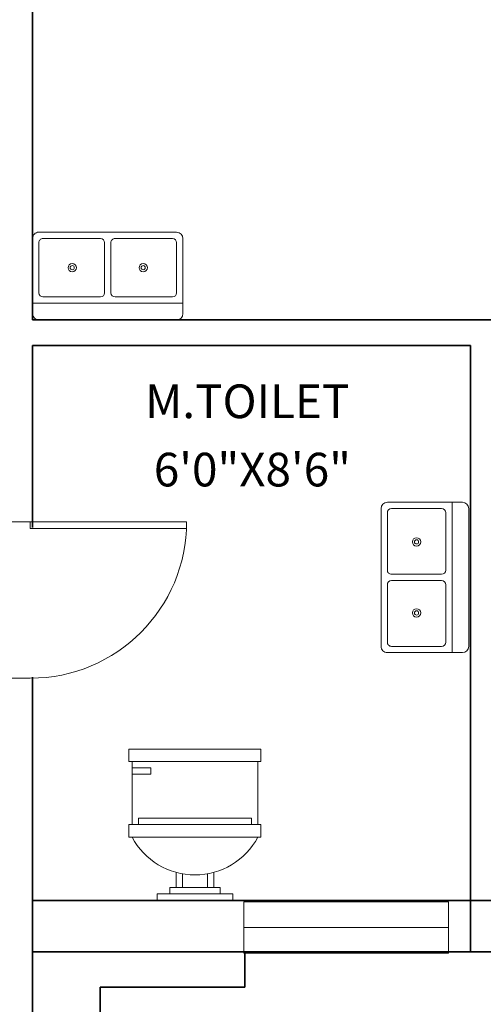
# Model space of a CAD drawing. Units: millimetres. Extents: x 27017497 to 27018854, y 7058029 to 7059154.
# Tile 30 of 91: x 27017804 to 27017886, y 7058124 to 7058297. Entities that reach past the tile are written whole.
import ezdxf

# ---------------------------------------------------------------- set-up
doc = ezdxf.new("R2010")
doc.units = ezdxf.units.MM
for name, color, linetype, lineweight in [('A-ANNO-DIMS', 2, 'Continuous', 18), ('A-AREA-IDEN', 7, 'Continuous', 18), ('A-DOOR', 4, 'Continuous', 20), ('A-FLOR-FIXT', 9, 'Continuous', 18), ('A-GLAZ', 4, 'Continuous', 18), ('A-WALL', 7, 'Continuous', 35)]:
    doc.layers.add(name, color=color, linetype=linetype, lineweight=lineweight)
doc.styles.get("Standard").update_dxf_attribs({"font": 'arial.ttf'})
doc.dimstyles.get("Standard").update_dxf_attribs({"dimtxt": 0.18, "dimasz": 0.18, "dimexe": 0.18, "dimexo": 0.0625, "dimgap": 0.09, "dimtad": 0, "dimtih": 1, "dimtoh": 1, "dimdec": 4, "dimzin": 0, "dimdsep": 46, "dimtxsty": 'Standard', "dimcen": 0.09, "dimadec": 0, "dimazin": 0, "dimtfac": 1, "dimtdec": 4, "dimtofl": 0, "dimtmove": 0, "dimatfit": 3, "dimfxl": 1, "dimtolj": 1, "dimtzin": 0, "dimarcsym": 0})

# ---------------------------------------------------------------- blocks, each defined once
blk = doc.blocks.new('*U2')
for p, q in [((0, 0), (0, -6)), ((40, 0), (40, -6))]:
    blk.add_line(p, q)
blk.add_lwpolyline([(0, 0), (0, 40), (1.75, 40), (1.75, 0)], close=True)
blk.add_arc((0, 0), 40, 0, 90)
blk = doc.blocks.new('*U6')
for p, q in [((-10, 22), (-10, 12)), ((10, 12), (10, 22)), ((-10, 21), (-7, 21)), ((-7, 21), (-7, 20)), ((-7, 20), (-10, 20)), ((9, 13), (-9, 13)), ((-9, 13), (-9, 12)), ((9, 12), (9, 13)), ((10.5, 12), (-10.5, 12)), ((-10.5, 10), (-10.5, 12)), ((10.5, 12), (10.5, 10)), ((10.5, 10), (-10.5, 10)), ((-3, 4.4065), (-3, 2)), ((-2, 2), (-2, 4.1658)), ((2, 4.1658), (2, 2)), ((3, 2), (3, 4.4065)), ((4, 2), (-4, 2)), ((-4, 2), (-4, 1)), ((4, 1), (4, 2))]:
    blk.add_line(p, q)
for points in [[(10.5, 22), (10.5, 24), (-10.5, 24), (-10.5, 22)], [(6, 0), (6, 1), (-6, 1), (-6, 0)]]:
    blk.add_lwpolyline(points, close=True)
blk.add_arc((0, 15.3333), 11.3333, 208.0725, 331.9275)
blk = doc.blocks.new('Sink-double - 36 in top')
for p, q in [((-18, -4), (18, -4)), ((-0.75, -18.5), (-0.75, -6.5)), ((0.75, -6.5), (0.75, -18.5))]:
    blk.add_line(p, q)
for points in [[(-16.5, 0), (16.5, 0)], [(-18, -19.5), (-18, -1.5)], [(18, -1.5), (18, -19.5)], [(-16.5, -18.5), (-16.5, -6.5)], [(-15.5, -5.5), (-1.75, -5.5)], [(1.75, -5.5), (15.5, -5.5)], [(16.5, -6.5), (16.5, -18.5)], [(16.5, -21), (-16.5, -21)], [(-1.75, -19.5), (-15.5, -19.5)], [(15.5, -19.5), (1.75, -19.5)]]:
    blk.add_lwpolyline(points)
for centre, radius in [((-8.5, -12.5), 1), ((8.5, -12.5), 1), ((-8.5, -12.5), 0.5), ((8.5, -12.5), 0.5)]:
    blk.add_circle(centre, radius)
for centre, radius, start, end in [((-16.5, -1.5), 1.5, 90, 180), ((16.5, -1.5), 1.5, 0, 90), ((-15.5, -6.5), 1, 90, 180), ((-1.75, -6.5), 1, 0, 90), ((1.75, -6.5), 1, 90, 180), ((15.5, -6.5), 1, 0, 90), ((-15.5, -18.5), 1, 180, 270), ((-1.75, -18.5), 1, 270, 0), ((1.75, -18.5), 1, 180, 270), ((15.5, -18.5), 1, 270, 0), ((-16.5, -19.5), 1.5, 180, 270), ((16.5, -19.5), 1.5, 270, 0)]:
    blk.add_arc(centre, radius, start, end)
blk = doc.blocks.new('WINDOW-SINGLE-LIGHT')
blk.add_lwpolyline([(36, 4.5), (36, 0), (0, 0), (0, 9), (36, 9), (36, 4.5), (0, 4.5)])
blk = doc.blocks.new('*D47')
at = {"layer": 'A-ANNO-DIMS', "color": 0, "lineweight": -2, "transparency": 16777216}
for p, q in [((27017561.17, 7058294.35), (27017561.17, 7058028.6)), ((27018790.61, 7058294.35), (27018790.61, 7058028.6)), ((27017561.35, 7058028.78), (27018175.43, 7058028.78)), ((27018790.43, 7058028.78), (27018176.34, 7058028.78))]:
    blk.add_line(p, q, dxfattribs=at)
at = {"layer": 'A-ANNO-DIMS', "color": 0, "transparency": 16777216}
for points in [[(27017561.35, 7058028.81), (27017561.35, 7058028.75), (27017561.17, 7058028.78)], [(27018790.43, 7058028.81), (27018790.43, 7058028.75), (27018790.61, 7058028.78)]]:
    blk.add_solid(points, dxfattribs=at)
at = {"layer": 'Defpoints', "color": 0, "transparency": 16777216}
for p in [(27017561.17, 7058294.41), (27018790.61, 7058294.41), (27018790.61, 7058028.78)]:
    blk.add_point(p, dxfattribs=at)
at = {"layer": 'A-ANNO-DIMS', "color": 0, "transparency": 16777216, "insert": (27018175.89, 7058028.78), "char_height": 0.18, "attachment_point": 5}
blk.add_mtext('\\A1;1229.4', dxfattribs=at)
blk = doc.blocks.new('*D48')
at = {"layer": 'A-ANNO-DIMS', "color": 0, "lineweight": -2, "transparency": 16777216}
for p, q in [((27018463.5, 7058622.91), (27017497.54, 7058622.91)), ((27017497.72, 7058622.73), (27017497.72, 7058357.75)), ((27017497.72, 7058092.41), (27017497.72, 7058357.39)), ((27018555.13, 7058092.23), (27017497.54, 7058092.23))]:
    blk.add_line(p, q, dxfattribs=at)
at = {"layer": 'A-ANNO-DIMS', "color": 0, "transparency": 16777216}
for points in [[(27017497.69, 7058622.73), (27017497.75, 7058622.73), (27017497.72, 7058622.91)], [(27017497.69, 7058092.41), (27017497.75, 7058092.41), (27017497.72, 7058092.23)]]:
    blk.add_solid(points, dxfattribs=at)
at = {"layer": 'Defpoints', "color": 0, "transparency": 16777216}
for p in [(27018463.56, 7058622.91), (27017497.72, 7058092.23), (27018555.19, 7058092.23)]:
    blk.add_point(p, dxfattribs=at)
at = {"layer": 'A-ANNO-DIMS', "color": 0, "transparency": 16777216, "insert": (27017497.72, 7058357.57), "char_height": 0.18, "attachment_point": 5}
blk.add_mtext('\\A1;530.7', dxfattribs=at)

msp = doc.modelspace()

# ---------------------------------------------------------------- linework, layer by layer
at = {"layer": 'A-WALL'}
for p, q in [((27017806.666, 7058298.912), (27017806.666, 7058243.912)), ((27017806.666, 7058243.912), (27017888.166, 7058243.912)), ((27017806.666, 7058239.412), (27017806.666, 7058207.442)), ((27017806.666, 7058239.412), (27017883.666, 7058239.412)), ((27017883.666, 7058239.412), (27017883.666, 7058202.912)), ((27017883.666, 7058202.912), (27017883.666, 7058132.912)), ((27017806.666, 7058181.164), (27017806.666, 7058094.141)), ((27017806.666, 7058141.912), (27017883.666, 7058141.912)), ((27017883.666, 7058141.912), (27018032.166, 7058141.912)), ((27017806.666, 7058132.912), (27017883.666, 7058132.912)), ((27017806.666, 7058132.912), (27017883.666, 7058132.912)), ((27017844.009, 7058126.681), (27017844.009, 7058132.822)), ((27017883.666, 7058132.912), (27018041.166, 7058132.912)), ((27017818.555, 7058094.141), (27017818.555, 7058126.681)), ((27017818.555, 7058126.681), (27017844.009, 7058126.681))]:
    msp.add_line(p, q, dxfattribs=at)

# ---------------------------------------------------------------- block references
at = {"layer": 'A-DOOR', "xscale": 0.6870473523349573, "yscale": 0.6870473523349573, "zscale": 0.6870473523349573, "rotation": 270}
msp.add_blockref('*U2', (27017806.287, 7058208.446), dxfattribs=at)
at = {"layer": 'A-FLOR-FIXT', "xscale": 0.7340308267416257, "yscale": 0.7340308267416257, "zscale": 0.7340308267416257}
for p, rotation in [((27017819.887, 7058243.912), 180), ((27017883.357, 7058198.673), 270)]:
    msp.add_blockref('Sink-double - 36 in top', p, dxfattribs=dict(at, rotation=rotation))
at = {"layer": 'A-FLOR-FIXT', "xscale": 1.105119395603938, "yscale": 1.105119395603938, "zscale": 1.105119395603938}
msp.add_blockref('*U6', (27017835.226, 7058141.991), dxfattribs=at)
at = {"layer": 'A-GLAZ'}
msp.add_blockref('WINDOW-SINGLE-LIGHT', (27017843.8, 7058132.679), dxfattribs=at)

# ---------------------------------------------------------------- texts
at = {"layer": 'A-ANNO-DIMS'}
msp.add_text('6\'0"X8\'6"', height=5.9118, dxfattribs=at).set_placement((27017827.992, 7058214.659))
at = {"layer": 'A-AREA-IDEN'}
msp.add_text('M.TOILET', height=5.9118, dxfattribs=at).set_placement((27017826.457, 7058226.657))

# ---------------------------------------------------------------- dimensions: what is measured, and where the dimension line sits
at = {"layer": 'A-ANNO-DIMS'}
dim = msp.add_linear_dim(base=(27017497.716, 7058092.23), p1=(27018463.561, 7058622.912), p2=(27018555.192, 7058092.23), angle=90, dimstyle='Standard', override={"dimdec": 1, "dimlfac": 1, "dimrnd": 0, "dimzin": 0, "dimdsep": 46, "dimlunit": 2}, dxfattribs=at)
dim.commit()
dim.dimension.update_dxf_attribs({"geometry": '*D48', "text_midpoint": (27017497.716, 7058357.571)})
dim = msp.add_linear_dim(base=(27018790.606, 7058028.78), p1=(27017561.166, 7058294.412), p2=(27018790.606, 7058294.412), dimstyle='Standard', override={"dimdec": 1, "dimlfac": 1, "dimrnd": 0, "dimzin": 0, "dimdsep": 46, "dimlunit": 2}, dxfattribs=at)
dim.commit()
dim.dimension.update_dxf_attribs({"geometry": '*D47', "text_midpoint": (27018175.886, 7058028.78)})

doc.saveas('drawing.dxf')
